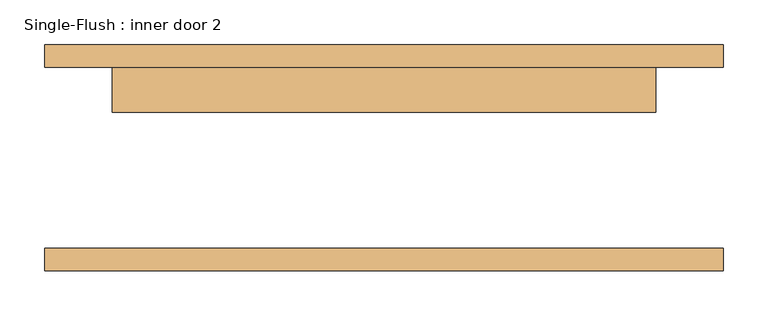
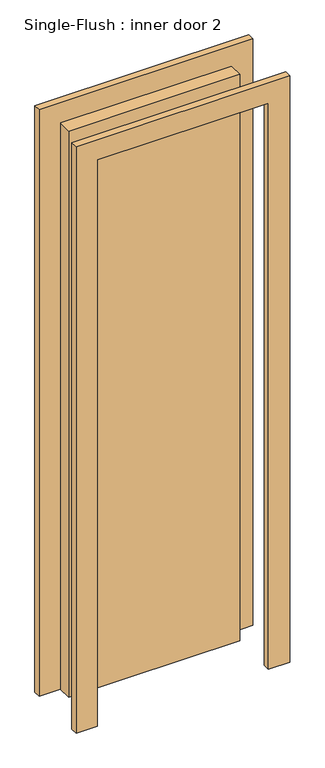
"""IFC4 building model written with IfcOpenShell, lengths in millimetres: door geometry, Single-Flush : inner door 2."""

from ifc_helpers import new_model, si_unit, frame, origin, origin_with_axes, place, context, project, spatial, polyline, outline, extrude, source, transform, mapped, element, save


def single_flush_inner_door_2_89112ad5(model_context):
    return source(origin(), model_context, "Body", "SweptSolid", [
        extrude(outline(polyline([(2209.8, -381.0), (0.0, -381.0), (0.0, -304.8), (2133.6, -304.8), (2133.6, 304.8), (0.0, 304.8), (0.0, 381.0), (2209.8, 381.0), (2209.8, -381.0)])), frame((0.0, 101.6, 0.0), z_axis=(0.0, 1.0, 0.0), x_axis=(0.0, 0.0, 1.0)), (0.0, 0.0, 1.0), 25.4),
        extrude(outline(polyline([(2209.8, 381.0), (2209.8, -381.0), (0.0, -381.0), (0.0, -304.8), (2133.6, -304.8), (2133.6, 304.8), (0.0, 304.8), (0.0, 381.0), (2209.8, 381.0)])), frame((0.0, -127.0, 0.0), z_axis=(0.0, 1.0, 0.0), x_axis=(0.0, 0.0, 1.0)), (0.0, 0.0, 1.0), 25.4),
        extrude(outline(polyline([(304.8, 50.8), (-304.8, 50.8), (-304.8, 101.6), (304.8, 101.6), (304.8, 50.8)])), origin_with_axes(), (0.0, 0.0, 1.0), 2133.6),
    ])


if __name__ == "__main__":
    model = new_model("IFC4")
    model_context = context("Model", 3, world=origin())
    ifc_project = project(units=[si_unit("LENGTHUNIT", "METRE", prefix="MILLI")], contexts=[model_context])
    site = spatial("IfcSite", under=ifc_project)
    building = spatial("IfcBuilding", under=site)
    placement = place(None, origin())
    single_flush_inner_door_2_shape = single_flush_inner_door_2_89112ad5(model_context)
    element("IfcDoor", 1, ObjectType="Single-Flush : inner door 2", at=placement, inside=building, context=model_context, shape_type="MappedRepresentation", body=[
        mapped(single_flush_inner_door_2_shape, transform((0.0, 0.0, 0.0), x_axis=(1.0, 0.0, 0.0), y_axis=(0.0, 1.0, 0.0), z_axis=(0.0, 0.0, 1.0))),
    ])
    save(model, "model.ifc")

# Revit data of these elements
# Type "Single-Flush : inner door 2"
#   Type Mark = "8"
#   Construction Type Id = "MDOOR"
#   Assembly Code = "C1020"
#   Analytic Construction = "Metal"
#   Thickness = 0' - 2"
#   Heat Transfer Coefficient (U) = 0.651978 BTU/(h·ft²·°F)
#   Height = 7' - 0"
#   Trim Projection Ext = 0' - 1"
#   Trim Projection Int = 0' - 1"
#   Trim Width = 0' - 3"
#   Width = 2' - 0"
#   Define Thermal Properties by = 1
#   Door Material = Door - Panel
#   Frame Material = Door - Frame
#   Visual Light Transmittance = 0
#   Solar Heat Gain Coefficient = 0
#   Function = (empty or 0)
#   Wall Closure = (empty or 0)
# Element 1 (IfcDoor, "Single-Flush : inner door 2")
#   Materials on its faces: "Door - Frame", "Door - Panel"
# Materials
#   "Door - Panel": class "Wood", colour RGB 210 159 95, transparency 0
#   "Door - Frame": colour RGB 118 70 51, transparency 0
